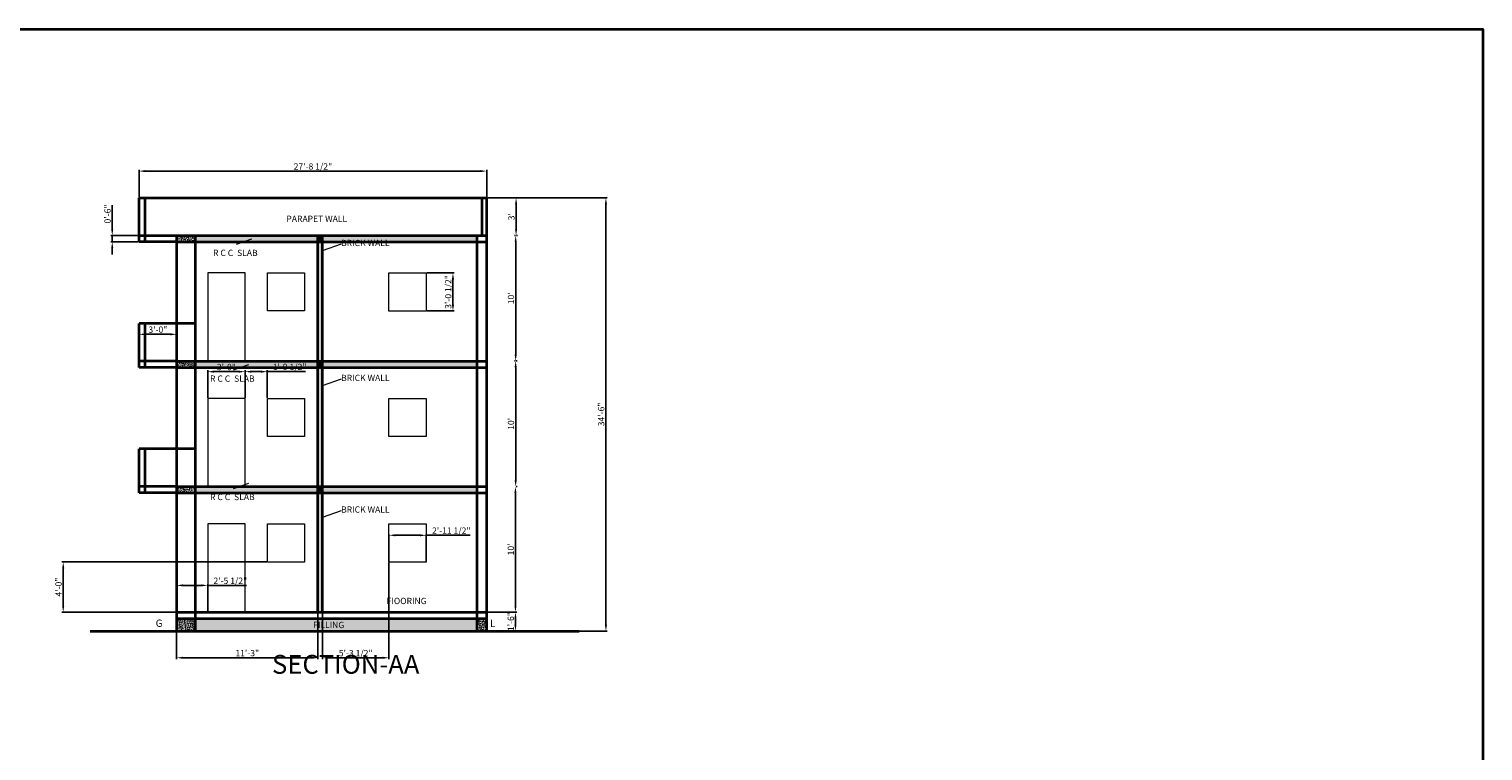
# Model space of a CAD drawing. Units: millimetres. Extents: x 50579 to 52843, y 62224 to 63803.
# Tile 5 of 5: x 51453 to 52843, y 63113 to 63803. Entities that reach past the tile are written whole.
import ezdxf

# ---------------------------------------------------------------- set-up
doc = ezdxf.new("R2010")
doc.units = ezdxf.units.MM
for name, color, linetype, lineweight in [('A-ANNO-DIMS', 2, 'Continuous', 18), ('A-ANNO-SYMB', 6, 'Continuous', 18), ('A-ANNO-TEXT', 6, 'Continuous', 18), ('A-ANNO-TITL', 4, 'Continuous', 25), ('A-ANNO-TTLB', 7, 'Continuous', 35), ('A-SECT', 7, 'Continuous', 35), ('A-SECT-OPEN', 7, 'Continuous', 18), ('A-SECT-PATT', 251, 'Continuous', 13)]:
    doc.layers.add(name, color=color, linetype=linetype, lineweight=lineweight)
doc.styles.get("Standard").update_dxf_attribs({"font": 'arial.ttf'})
doc.dimstyles.new('ISO-25', dxfattribs={"dimtxt": 6, "dimasz": 6, "dimexe": 1.25, "dimexo": 0.625, "dimtad": 1, "dimdec": 0, "dimlunit": 3, "dimtxsty": 'Standard', "dimcen": 2.5, "dimadec": 0, "dimazin": 0, "dimtfac": 1, "dimtdec": 0, "dimtmove": 0, "dimatfit": 3, "dimfxl": 1, "dimarcsym": 0})

# ---------------------------------------------------------------- blocks, each defined once
blk = doc.blocks.new('*D16')
at = {"layer": 'A-ANNO-DIMS', "color": 0, "lineweight": -2, "transparency": 16777216}
for p, q in [((51891, 63245.3), (51919.1, 63245.3)), ((51917.9, 63233.3), (51917.9, 63239.3)), ((51891, 63227.3), (51919.1, 63227.3))]:
    blk.add_line(p, q, dxfattribs=at)
at = {"layer": 'A-ANNO-DIMS', "color": 0, "transparency": 16777216}
for points in [[(51916.9, 63239.3), (51918.9, 63239.3), (51917.9, 63245.3)], [(51916.9, 63233.3), (51918.9, 63233.3), (51917.9, 63227.3)]]:
    blk.add_solid(points, dxfattribs=at)
at = {"layer": 'Defpoints', "color": 0, "transparency": 16777216}
for p in [(51890.4, 63245.3), (51917.9, 63245.3), (51890.4, 63227.3)]:
    blk.add_point(p, dxfattribs=at)
at = {"layer": 'A-ANNO-DIMS', "color": 0, "transparency": 16777216, "insert": (51914.2, 63236.3), "char_height": 6, "attachment_point": 5, "rotation": 90}
blk.add_mtext('1\'-6"', dxfattribs=at)
blk = doc.blocks.new('*D17')
at = {"layer": 'A-ANNO-DIMS', "color": 0, "lineweight": -2, "transparency": 16777216}
for p, q in [((51917.9, 63251.3), (51917.9, 63359.3)), ((51918.5, 63365.3), (51919.1, 63365.3)), ((51918.5, 63245.3), (51919.1, 63245.3))]:
    blk.add_line(p, q, dxfattribs=at)
at = {"layer": 'A-ANNO-DIMS', "color": 0, "transparency": 16777216}
for points in [[(51916.9, 63359.3), (51918.9, 63359.3), (51917.9, 63365.3)], [(51916.9, 63251.3), (51918.9, 63251.3), (51917.9, 63245.3)]]:
    blk.add_solid(points, dxfattribs=at)
at = {"layer": 'Defpoints', "color": 0, "transparency": 16777216}
for p in [(51917.9, 63365.3), (51917.9, 63365.3), (51917.9, 63245.3)]:
    blk.add_point(p, dxfattribs=at)
at = {"layer": 'A-ANNO-DIMS', "color": 0, "transparency": 16777216, "insert": (51914.2, 63305.3), "char_height": 6, "attachment_point": 5, "rotation": 90}
blk.add_mtext("10'", dxfattribs=at)
blk = doc.blocks.new('*D18')
at = {"layer": 'A-ANNO-DIMS', "color": 0, "lineweight": -2, "transparency": 16777216}
for p, q in [((51918.5, 63485.4), (51919.4, 63485.4)), ((51918.1, 63371.3), (51918.1, 63479.4)), ((51918.5, 63365.3), (51919.4, 63365.3))]:
    blk.add_line(p, q, dxfattribs=at)
at = {"layer": 'A-ANNO-DIMS', "color": 0, "transparency": 16777216}
for points in [[(51917.1, 63479.4), (51919.1, 63479.4), (51918.1, 63485.4)], [(51917.1, 63371.3), (51919.1, 63371.3), (51918.1, 63365.3)]]:
    blk.add_solid(points, dxfattribs=at)
at = {"layer": 'Defpoints', "color": 0, "transparency": 16777216}
for p in [(51917.9, 63485.4), (51918.1, 63485.4), (51917.9, 63365.3)]:
    blk.add_point(p, dxfattribs=at)
at = {"layer": 'A-ANNO-DIMS', "color": 0, "transparency": 16777216, "insert": (51914.4, 63425.3), "char_height": 6, "attachment_point": 5, "rotation": 90}
blk.add_mtext("10'", dxfattribs=at)
blk = doc.blocks.new('*D19')
at = {"layer": 'A-ANNO-DIMS', "color": 0, "lineweight": -2, "transparency": 16777216}
for p, q in [((51917.9, 63605.3), (51916.9, 63605.3)), ((51918.1, 63491.4), (51918.1, 63599.3)), ((51917.9, 63485.4), (51916.9, 63485.4))]:
    blk.add_line(p, q, dxfattribs=at)
at = {"layer": 'A-ANNO-DIMS', "color": 0, "transparency": 16777216}
for points in [[(51917.1, 63599.3), (51919.1, 63599.3), (51918.1, 63605.3)], [(51917.1, 63491.4), (51919.1, 63491.4), (51918.1, 63485.4)]]:
    blk.add_solid(points, dxfattribs=at)
at = {"layer": 'Defpoints', "color": 0, "transparency": 16777216}
for p in [(51918.1, 63605.3), (51918.5, 63605.3), (51918.5, 63485.4)]:
    blk.add_point(p, dxfattribs=at)
at = {"layer": 'A-ANNO-DIMS', "color": 0, "transparency": 16777216, "insert": (51914.4, 63545.3), "char_height": 6, "attachment_point": 5, "rotation": 90}
blk.add_mtext("10'", dxfattribs=at)
blk = doc.blocks.new('*D20')
at = {"layer": 'A-ANNO-DIMS', "color": 0, "lineweight": -2, "transparency": 16777216}
for p, q in [((51918.8, 63641.3), (51919.7, 63641.3)), ((51918.5, 63611.3), (51918.5, 63635.3)), ((51918.8, 63605.3), (51919.7, 63605.3))]:
    blk.add_line(p, q, dxfattribs=at)
at = {"layer": 'A-ANNO-DIMS', "color": 0, "transparency": 16777216}
for points in [[(51917.5, 63635.3), (51919.5, 63635.3), (51918.5, 63641.3)], [(51917.5, 63611.3), (51919.5, 63611.3), (51918.5, 63605.3)]]:
    blk.add_solid(points, dxfattribs=at)
at = {"layer": 'Defpoints', "color": 0, "transparency": 16777216}
for p in [(51918.1, 63641.3), (51918.5, 63641.3), (51918.1, 63605.3)]:
    blk.add_point(p, dxfattribs=at)
at = {"layer": 'A-ANNO-DIMS', "color": 0, "transparency": 16777216, "insert": (51914.8, 63623.3), "char_height": 6, "attachment_point": 5, "rotation": 90}
blk.add_mtext("3'", dxfattribs=at)
blk = doc.blocks.new('*D47')
at = {"layer": 'A-ANNO-DIMS', "color": 0, "lineweight": -2, "transparency": 16777216}
for p, q in [((51557.9, 63641.9), (51557.9, 63668.1)), ((51563.9, 63666.9), (51884.4, 63666.9)), ((51890.4, 63641.9), (51890.4, 63668.1))]:
    blk.add_line(p, q, dxfattribs=at)
at = {"layer": 'A-ANNO-DIMS', "color": 0, "transparency": 16777216}
for points in [[(51563.9, 63667.9), (51563.9, 63665.9), (51557.9, 63666.9)], [(51884.4, 63667.9), (51884.4, 63665.9), (51890.4, 63666.9)]]:
    blk.add_solid(points, dxfattribs=at)
at = {"layer": 'Defpoints', "color": 0, "transparency": 16777216}
for p in [(51890.4, 63666.9), (51557.9, 63641.3), (51890.4, 63641.3)]:
    blk.add_point(p, dxfattribs=at)
at = {"layer": 'A-ANNO-DIMS', "color": 0, "transparency": 16777216, "insert": (51724.2, 63670.6), "char_height": 6, "attachment_point": 5}
blk.add_mtext('27\'-8 1/2"', dxfattribs=at)
blk = doc.blocks.new('*D48')
at = {"layer": 'A-ANNO-DIMS', "color": 0, "lineweight": -2, "transparency": 16777216}
for p, q in [((51891, 63641.3), (52005.7, 63641.3)), ((52004.4, 63233.3), (52004.4, 63635.3)), ((51891, 63227.3), (52005.7, 63227.3))]:
    blk.add_line(p, q, dxfattribs=at)
at = {"layer": 'A-ANNO-DIMS', "color": 0, "transparency": 16777216}
for points in [[(52003.4, 63635.3), (52005.4, 63635.3), (52004.4, 63641.3)], [(52003.4, 63233.3), (52005.4, 63233.3), (52004.4, 63227.3)]]:
    blk.add_solid(points, dxfattribs=at)
at = {"layer": 'Defpoints', "color": 0, "transparency": 16777216}
for p in [(51890.4, 63641.3), (52004.4, 63641.3), (51890.4, 63227.3)]:
    blk.add_point(p, dxfattribs=at)
at = {"layer": 'A-ANNO-DIMS', "color": 0, "transparency": 16777216, "insert": (52000.7, 63434.3), "char_height": 6, "attachment_point": 5, "rotation": 90}
blk.add_mtext('34\'-6"', dxfattribs=at)
blk = doc.blocks.new('*D58')
at = {"layer": 'A-ANNO-DIMS', "color": 0, "lineweight": -2, "transparency": 16777216}
for p, q in [((51728.9, 63244.7), (51728.9, 63200.4)), ((51593.9, 63226.7), (51593.9, 63200.4)), ((51599.9, 63201.7), (51722.9, 63201.7))]:
    blk.add_line(p, q, dxfattribs=at)
at = {"layer": 'A-ANNO-DIMS', "color": 0, "transparency": 16777216}
for points in [[(51599.9, 63202.7), (51599.9, 63200.7), (51593.9, 63201.7)], [(51722.9, 63202.7), (51722.9, 63200.7), (51728.9, 63201.7)]]:
    blk.add_solid(points, dxfattribs=at)
at = {"layer": 'Defpoints', "color": 0, "transparency": 16777216}
for p in [(51728.9, 63245.3), (51593.9, 63227.3), (51728.9, 63201.7)]:
    blk.add_point(p, dxfattribs=at)
at = {"layer": 'A-ANNO-DIMS', "color": 0, "transparency": 16777216, "insert": (51661.4, 63205.4), "char_height": 6, "attachment_point": 5}
blk.add_mtext('11\'-3"', dxfattribs=at)
blk = doc.blocks.new('*D59')
at = {"layer": 'A-ANNO-DIMS', "color": 0, "lineweight": -2, "transparency": 16777216}
for p, q in [((51557.9, 63485.9), (51557.9, 63512.1)), ((51563.9, 63510.9), (51587.9, 63510.9)), ((51593.9, 63485.9), (51593.9, 63512.1))]:
    blk.add_line(p, q, dxfattribs=at)
at = {"layer": 'A-ANNO-DIMS', "color": 0, "transparency": 16777216}
for points in [[(51563.9, 63511.9), (51563.9, 63509.9), (51557.9, 63510.9)], [(51587.9, 63511.9), (51587.9, 63509.9), (51593.9, 63510.9)]]:
    blk.add_solid(points, dxfattribs=at)
at = {"layer": 'Defpoints', "color": 0, "transparency": 16777216}
for p in [(51593.9, 63510.9), (51557.9, 63485.3), (51593.9, 63485.3)]:
    blk.add_point(p, dxfattribs=at)
at = {"layer": 'A-ANNO-DIMS', "color": 0, "transparency": 16777216, "insert": (51575.9, 63514.6), "char_height": 6, "attachment_point": 5}
blk.add_mtext('3\'-0"', dxfattribs=at)
blk = doc.blocks.new('*D60')
at = {"layer": 'A-ANNO-DIMS', "color": 0, "lineweight": -2, "transparency": 16777216}
for p, q in [((51593.9, 63245.9), (51593.9, 63272.1)), ((51599.9, 63270.9), (51617.6, 63270.9)), ((51623.6, 63245.9), (51623.6, 63272.1)), ((51623.6, 63270.9), (51660.8, 63270.9))]:
    blk.add_line(p, q, dxfattribs=at)
at = {"layer": 'A-ANNO-DIMS', "color": 0, "transparency": 16777216}
for points in [[(51599.9, 63271.9), (51599.9, 63269.9), (51593.9, 63270.9)], [(51617.6, 63271.9), (51617.6, 63269.9), (51623.6, 63270.9)]]:
    blk.add_solid(points, dxfattribs=at)
at = {"layer": 'Defpoints', "color": 0, "transparency": 16777216}
for p in [(51623.6, 63270.9), (51593.9, 63245.3), (51623.6, 63245.3)]:
    blk.add_point(p, dxfattribs=at)
at = {"layer": 'A-ANNO-DIMS', "color": 0, "transparency": 16777216, "insert": (51645.2, 63274.6), "char_height": 6, "attachment_point": 5}
blk.add_mtext('2\'-5 1/2"', dxfattribs=at)
blk = doc.blocks.new('*D61')
at = {"layer": 'A-ANNO-DIMS', "color": 0, "lineweight": -2, "transparency": 16777216}
for p, q in [((51623.6, 63450.3), (51623.6, 63476.5)), ((51629.6, 63475.2), (51653.3, 63475.2)), ((51659.3, 63450.3), (51659.3, 63476.5))]:
    blk.add_line(p, q, dxfattribs=at)
at = {"layer": 'A-ANNO-DIMS', "color": 0, "transparency": 16777216}
for points in [[(51629.6, 63476.2), (51629.6, 63474.2), (51623.6, 63475.2)], [(51653.3, 63476.2), (51653.3, 63474.2), (51659.3, 63475.2)]]:
    blk.add_solid(points, dxfattribs=at)
at = {"layer": 'Defpoints', "color": 0, "transparency": 16777216}
for p in [(51659.3, 63475.2), (51623.6, 63449.6), (51659.3, 63449.6)]:
    blk.add_point(p, dxfattribs=at)
at = {"layer": 'A-ANNO-DIMS', "color": 0, "transparency": 16777216, "insert": (51641.4, 63478.9), "char_height": 6, "attachment_point": 5}
blk.add_mtext('3\'-0"', dxfattribs=at)
blk = doc.blocks.new('*D62')
at = {"layer": 'A-ANNO-DIMS', "color": 0, "lineweight": -2, "transparency": 16777216}
for p, q in [((51659.3, 63450.3), (51659.3, 63476.5)), ((51665.3, 63475.2), (51674.6, 63475.2)), ((51680.6, 63450.3), (51680.6, 63476.5)), ((51680.6, 63475.2), (51717.2, 63475.2))]:
    blk.add_line(p, q, dxfattribs=at)
at = {"layer": 'A-ANNO-DIMS', "color": 0, "transparency": 16777216}
for points in [[(51665.3, 63476.2), (51665.3, 63474.2), (51659.3, 63475.2)], [(51674.6, 63476.2), (51674.6, 63474.2), (51680.6, 63475.2)]]:
    blk.add_solid(points, dxfattribs=at)
at = {"layer": 'Defpoints', "color": 0, "transparency": 16777216}
for p in [(51680.6, 63475.2), (51659.3, 63449.6), (51680.6, 63449.6)]:
    blk.add_point(p, dxfattribs=at)
at = {"layer": 'A-ANNO-DIMS', "color": 0, "transparency": 16777216, "insert": (51701.9, 63479), "char_height": 6, "attachment_point": 5}
blk.add_mtext('1\'-9 1/2"', dxfattribs=at)
blk = doc.blocks.new('*D63')
at = {"layer": 'A-ANNO-DIMS', "color": 0, "lineweight": -2, "transparency": 16777216}
for p, q in [((51796.9, 63292.6), (51796.9, 63200.4)), ((51733.4, 63244.7), (51733.4, 63200.4)), ((51739.4, 63201.7), (51790.9, 63201.7))]:
    blk.add_line(p, q, dxfattribs=at)
at = {"layer": 'A-ANNO-DIMS', "color": 0, "transparency": 16777216}
for points in [[(51739.4, 63202.7), (51739.4, 63200.7), (51733.4, 63201.7)], [(51790.9, 63202.7), (51790.9, 63200.7), (51796.9, 63201.7)]]:
    blk.add_solid(points, dxfattribs=at)
at = {"layer": 'Defpoints', "color": 0, "transparency": 16777216}
for p in [(51796.9, 63293.2), (51733.4, 63245.3), (51796.9, 63201.7)]:
    blk.add_point(p, dxfattribs=at)
at = {"layer": 'A-ANNO-DIMS', "color": 0, "transparency": 16777216, "insert": (51765.1, 63205.4), "char_height": 6, "attachment_point": 5}
blk.add_mtext('5\'-3 1/2"', dxfattribs=at)
blk = doc.blocks.new('*D64')
at = {"layer": 'A-ANNO-DIMS', "color": 0, "lineweight": -2, "transparency": 16777216}
for p, q in [((51796.9, 63293.8), (51796.9, 63320)), ((51802.9, 63318.8), (51826.5, 63318.8)), ((51832.5, 63293.8), (51832.5, 63320)), ((51832.5, 63318.8), (51874.5, 63318.8))]:
    blk.add_line(p, q, dxfattribs=at)
at = {"layer": 'A-ANNO-DIMS', "color": 0, "transparency": 16777216}
for points in [[(51802.9, 63319.8), (51802.9, 63317.8), (51796.9, 63318.8)], [(51826.5, 63319.8), (51826.5, 63317.8), (51832.5, 63318.8)]]:
    blk.add_solid(points, dxfattribs=at)
at = {"layer": 'Defpoints', "color": 0, "transparency": 16777216}
for p in [(51832.5, 63318.8), (51796.9, 63293.2), (51832.5, 63293.2)]:
    blk.add_point(p, dxfattribs=at)
at = {"layer": 'A-ANNO-DIMS', "color": 0, "transparency": 16777216, "insert": (51856.5, 63322.5), "char_height": 6, "attachment_point": 5}
blk.add_mtext('2\'-11 1/2"', dxfattribs=at)
blk = doc.blocks.new('*D65')
at = {"layer": 'A-ANNO-DIMS', "color": 0, "lineweight": -2, "transparency": 16777216}
for p, q in [((51833.1, 63569.6), (51859.4, 63569.6)), ((51858.1, 63563.6), (51858.1, 63539.2)), ((51833.1, 63533.2), (51859.4, 63533.2))]:
    blk.add_line(p, q, dxfattribs=at)
at = {"layer": 'A-ANNO-DIMS', "color": 0, "transparency": 16777216}
for points in [[(51857.1, 63563.6), (51859.1, 63563.6), (51858.1, 63569.6)], [(51857.1, 63539.2), (51859.1, 63539.2), (51858.1, 63533.2)]]:
    blk.add_solid(points, dxfattribs=at)
at = {"layer": 'Defpoints', "color": 0, "transparency": 16777216}
for p in [(51832.5, 63569.6), (51832.5, 63533.2), (51858.1, 63533.2)]:
    blk.add_point(p, dxfattribs=at)
at = {"layer": 'A-ANNO-DIMS', "color": 0, "transparency": 16777216, "insert": (51854.4, 63551.4), "char_height": 6, "attachment_point": 5, "rotation": 90}
blk.add_mtext('3\'-0 1/2"', dxfattribs=at)
blk = doc.blocks.new('*D66')
at = {"layer": 'A-ANNO-DIMS', "color": 0, "lineweight": -2, "transparency": 16777216}
for p, q in [((51680, 63293.3), (51484.2, 63293.3)), ((51485.4, 63287.3), (51485.4, 63251.3)), ((51658.7, 63245.3), (51484.2, 63245.3))]:
    blk.add_line(p, q, dxfattribs=at)
at = {"layer": 'A-ANNO-DIMS', "color": 0, "transparency": 16777216}
for points in [[(51484.4, 63287.3), (51486.4, 63287.3), (51485.4, 63293.3)], [(51484.4, 63251.3), (51486.4, 63251.3), (51485.4, 63245.3)]]:
    blk.add_solid(points, dxfattribs=at)
at = {"layer": 'Defpoints', "color": 0, "transparency": 16777216}
for p in [(51680.6, 63293.3), (51485.4, 63245.3), (51659.3, 63245.3)]:
    blk.add_point(p, dxfattribs=at)
at = {"layer": 'A-ANNO-DIMS', "color": 0, "transparency": 16777216, "insert": (51481.7, 63269.3), "char_height": 6, "attachment_point": 5, "rotation": 90}
blk.add_mtext('4\'-0"', dxfattribs=at)
blk = doc.blocks.new('*D67')
at = {"layer": 'A-ANNO-DIMS', "color": 0, "lineweight": -2, "transparency": 16777216}
for p, q in [((51532.3, 63611.3), (51532.3, 63634.5)), ((51557.3, 63605.3), (51531.1, 63605.3)), ((51557.3, 63599.3), (51531.1, 63599.3)), ((51532.3, 63599.3), (51532.3, 63605.3)), ((51532.3, 63593.3), (51532.3, 63587.3))]:
    blk.add_line(p, q, dxfattribs=at)
at = {"layer": 'A-ANNO-DIMS', "color": 0, "transparency": 16777216}
for points in [[(51531.3, 63611.3), (51533.3, 63611.3), (51532.3, 63605.3)], [(51531.3, 63593.3), (51533.3, 63593.3), (51532.3, 63599.3)]]:
    blk.add_solid(points, dxfattribs=at)
at = {"layer": 'Defpoints', "color": 0, "transparency": 16777216}
for p in [(51532.3, 63605.3), (51557.9, 63605.3), (51557.9, 63599.3)]:
    blk.add_point(p, dxfattribs=at)
at = {"layer": 'A-ANNO-DIMS', "color": 0, "transparency": 16777216, "insert": (51528.6, 63625.9), "char_height": 6, "attachment_point": 5, "rotation": 90}
blk.add_mtext('0\'-6"', dxfattribs=at)

msp = doc.modelspace()

# ---------------------------------------------------------------- hatches: boundary and pattern name
at = {"layer": 'A-SECT-PATT'}
h = msp.add_hatch(dxfattribs=at)
h.set_pattern_fill('AR-CONC', color=256, scale=0.01)
h.paths.add_polyline_path([(51611.8, 63605.28), (51593.92, 63605.28), (51593.92, 63599.28), (51611.8, 63599.28)])
h = msp.add_hatch(dxfattribs=at)
h.set_pattern_fill('AR-CONC', color=256, scale=0.01)
h.paths.add_polyline_path([(51728.92, 63605.28), (51611.8, 63605.28), (51611.8, 63599.28), (51728.92, 63599.28)])
h = msp.add_hatch(dxfattribs=at)
h.set_pattern_fill('BRICK', color=256, scale=0.01)
h.paths.add_polyline_path([(51733.42, 63605.28), (51728.92, 63605.28), (51728.92, 63599.28), (51733.42, 63599.28)])
h = msp.add_hatch(dxfattribs=at)
h.set_pattern_fill('BRICK', color=256, scale=0.01)
h.paths.add_polyline_path([(51733.42, 63599.28), (51728.92, 63599.28), (51728.92, 63485.28), (51733.42, 63485.28)])
h = msp.add_hatch(dxfattribs=at)
h.set_pattern_fill('AR-CONC', color=256, scale=0.01)
h.paths.add_polyline_path([(51881.42, 63605.28), (51733.42, 63605.28), (51733.42, 63599.28), (51881.42, 63599.28)])
h = msp.add_hatch(dxfattribs=at)
h.set_pattern_fill('AR-CONC', color=256, scale=0.01)
h.paths.add_polyline_path([(51611.8, 63485.28), (51593.92, 63485.28), (51593.92, 63479.28), (51611.8, 63479.28)])
h = msp.add_hatch(dxfattribs=at)
h.set_pattern_fill('AR-CONC', color=256, scale=0.01)
h.paths.add_polyline_path([(51728.92, 63485.28), (51611.8, 63485.28), (51611.8, 63479.28), (51728.92, 63479.28)])
h = msp.add_hatch(dxfattribs=at)
h.set_pattern_fill('BRICK', color=256, scale=0.01)
h.paths.add_polyline_path([(51733.42, 63485.28), (51728.92, 63485.28), (51728.92, 63479.28), (51733.42, 63479.28)])
h = msp.add_hatch(dxfattribs=at)
h.set_pattern_fill('AR-CONC', color=256, scale=0.01)
h.paths.add_polyline_path([(51881.42, 63485.28), (51733.42, 63485.28), (51733.42, 63479.28), (51881.42, 63479.28)])
h = msp.add_hatch(dxfattribs=at)
h.set_pattern_fill('BRICK', color=256, scale=0.01)
h.paths.add_polyline_path([(51733.42, 63479.28), (51728.92, 63479.28), (51728.92, 63365.28), (51733.42, 63365.28)])
h = msp.add_hatch(dxfattribs=at)
h.set_pattern_fill('AR-CONC', color=256, scale=0.01)
h.paths.add_polyline_path([(51611.8, 63365.28), (51593.92, 63365.28), (51593.92, 63359.28), (51611.8, 63359.28)])
h = msp.add_hatch(dxfattribs=at)
h.set_pattern_fill('AR-CONC', color=256, scale=0.01)
h.paths.add_polyline_path([(51728.92, 63365.28), (51611.8, 63365.28), (51611.8, 63359.28), (51728.92, 63359.28)])
h = msp.add_hatch(dxfattribs=at)
h.set_pattern_fill('BRICK', color=256, scale=0.01)
h.paths.add_polyline_path([(51733.42, 63365.28), (51728.92, 63365.28), (51728.92, 63359.28), (51733.42, 63359.28)])
h = msp.add_hatch(dxfattribs=at)
h.set_pattern_fill('BRICK', color=256, scale=0.01)
h.paths.add_polyline_path([(51733.42, 63359.28), (51728.92, 63359.28), (51728.92, 63245.28), (51733.42, 63245.28)])
h = msp.add_hatch(dxfattribs=at)
h.set_pattern_fill('AR-CONC', color=256, scale=0.01)
h.paths.add_polyline_path([(51881.42, 63365.28), (51733.42, 63365.28), (51733.42, 63359.28), (51881.42, 63359.28)])
h = msp.add_hatch(dxfattribs=at)
h.set_pattern_fill('AR-CONC', color=256, scale=0.01)
h.paths.add_polyline_path([(51611.8, 63239.28), (51593.92, 63239.28), (51593.92, 63227.28), (51611.8, 63227.28)])
h = msp.add_hatch(dxfattribs=at)
h.set_pattern_fill('AR-CONC', color=256, scale=0.01)
h.paths.add_polyline_path([(51881.42, 63239.28), (51611.8, 63239.28), (51611.8, 63227.28), (51881.42, 63227.28)])
h = msp.add_hatch(dxfattribs=at)
h.set_pattern_fill('AR-CONC', color=256, scale=0.01)
h.paths.add_polyline_path([(51890.42, 63239.28), (51881.42, 63239.28), (51881.42, 63227.28), (51890.42, 63227.28)])

# ---------------------------------------------------------------- linework, layer by layer
at = {"layer": 'A-ANNO-TEXT'}
for p, q in [((51665.37, 63601.77), (51650.75, 63596.65)), ((51733.42, 63590.88), (51751.68, 63597.27)), ((51662.51, 63481.59), (51647.89, 63476.47)), ((51733.42, 63461.89), (51751.68, 63468.29)), ((51662.51, 63368.43), (51647.89, 63363.31)), ((51733.42, 63336.09), (51751.68, 63342.48))]:
    msp.add_line(p, q, dxfattribs=at)
at = {"layer": 'A-ANNO-TTLB'}
msp.add_lwpolyline([(50579.46, 63802.65), (52843.1, 63802.65), (52843.1, 62224.04), (50579.46, 62224.04)], close=True, dxfattribs=at)
at = {"layer": 'A-SECT'}
for p, q in [((51557.92, 63599.28), (51557.92, 63641.28)), ((51557.92, 63641.28), (51890.42, 63641.28)), ((51563.92, 63599.28), (51563.92, 63641.28)), ((51885.92, 63605.28), (51885.92, 63641.28)), ((51890.42, 63227.28), (51890.42, 63641.28)), ((51557.92, 63605.28), (51890.42, 63605.28)), ((51593.92, 63599.28), (51557.92, 63599.28)), ((51593.92, 63227.28), (51593.92, 63605.28)), ((51593.92, 63599.28), (51890.42, 63599.28)), ((51611.8, 63227.28), (51611.8, 63605.28)), ((51728.92, 63245.28), (51728.92, 63605.28)), ((51733.42, 63245.28), (51733.42, 63605.28)), ((51881.42, 63227.28), (51881.42, 63605.28)), ((51557.92, 63479.28), (51557.92, 63521.28)), ((51611.8, 63521.28), (51557.92, 63521.28)), ((51563.92, 63479.28), (51563.92, 63521.28)), ((51593.92, 63485.28), (51557.92, 63485.28)), ((51593.92, 63485.28), (51890.42, 63485.28)), ((51593.92, 63479.28), (51557.92, 63479.28)), ((51593.92, 63479.28), (51890.42, 63479.28)), ((51557.92, 63359.28), (51557.92, 63401.28)), ((51611.8, 63401.28), (51557.92, 63401.28)), ((51563.92, 63359.28), (51563.92, 63401.28)), ((51593.92, 63365.28), (51557.92, 63365.28)), ((51593.92, 63359.28), (51557.92, 63359.28)), ((51593.92, 63365.28), (51890.42, 63365.28)), ((51593.92, 63359.28), (51890.42, 63359.28)), ((51593.92, 63245.28), (51890.42, 63245.28)), ((51593.92, 63239.28), (51890.42, 63239.28)), ((51511.03, 63227.28), (51978.82, 63227.28))]:
    msp.add_line(p, q, dxfattribs=at)
at = {"layer": 'A-SECT-OPEN'}
for points in [[(51623.56, 63485.28), (51659.31, 63485.28), (51659.31, 63569.63), (51623.56, 63569.63)], [(51680.63, 63569.63), (51716.01, 63569.63), (51716.01, 63533.26), (51680.63, 63533.26)], [(51796.88, 63569.63), (51832.52, 63569.63), (51832.52, 63533.18), (51796.88, 63533.18)], [(51623.56, 63365.28), (51659.31, 63365.28), (51659.31, 63449.63), (51623.56, 63449.63)], [(51680.63, 63449.63), (51716.01, 63449.63), (51716.01, 63413.26), (51680.63, 63413.26)], [(51796.88, 63449.63), (51832.52, 63449.63), (51832.52, 63413.18), (51796.88, 63413.18)], [(51623.56, 63245.28), (51659.31, 63245.28), (51659.31, 63329.63), (51623.56, 63329.63)], [(51680.63, 63329.63), (51716.01, 63329.63), (51716.01, 63293.26), (51680.63, 63293.26)], [(51796.88, 63329.63), (51832.52, 63329.63), (51832.52, 63293.18), (51796.88, 63293.18)]]:
    msp.add_lwpolyline(points, close=True, dxfattribs=at)

# ---------------------------------------------------------------- texts
at = {"layer": 'A-ANNO-SYMB', "char_height": 7, "attachment_point": 1}
for s, insert in [('  G', (51569.56, 63238.26)), ('  L', (51889.22, 63238.04))]:
    msp.add_mtext_dynamic_manual_height_columns(s, width=13.8936, gutter_width=12.5, heights=[0], dxfattribs=dict(at, insert=insert))
at = {"layer": 'A-ANNO-TEXT', "char_height": 6, "attachment_point": 1}
for s, insert in [('    PARAPET WALL', (51691.47, 63624.29)), ('   BRICK WALL', (51745.63, 63601.21)), ('    R C C  SLAB', (51621.36, 63591.73)), ('    R C C  SLAB', (51618.5, 63471.55)), ('   BRICK WALL', (51745.63, 63472.23)), ('    R C C  SLAB', (51618.5, 63358.39)), ('   BRICK WALL', (51745.63, 63346.42)), ('    FIOORING', (51787.36, 63259.02)), ('    FILLING', (51717.07, 63236.08))]:
    msp.add_mtext_dynamic_manual_height_columns(s, width=88.9546, gutter_width=12.5, heights=[0], dxfattribs=dict(at, insert=insert))
at = {"layer": 'A-ANNO-TITL', "insert": (51674.06, 63204.47), "char_height": 18, "attachment_point": 1}
msp.add_mtext_dynamic_manual_height_columns('  SECTION-AA', width=341.9217, gutter_width=12.5, heights=[0], dxfattribs=at)

# ---------------------------------------------------------------- dimensions: what is measured, and where the dimension line sits
at = {"layer": 'A-ANNO-DIMS'}
for base, p1, p2, picture, middle in [((51890.42, 63666.88), (51557.92, 63641.28), (51890.42, 63641.28), '*D47', (51724.17, 63670.61)), ((51593.92, 63510.88), (51557.92, 63485.28), (51593.92, 63485.28), '*D59', (51575.92, 63514.57)), ((51659.3082, 63475.225), (51623.5577, 63449.625), (51659.3082, 63449.625), '*D61', (51641.433, 63478.9155)), ((51680.63, 63475.23), (51659.31, 63449.63), (51680.63, 63449.63), '*D62', (51701.93, 63478.95)), ((51832.52, 63318.78), (51796.88, 63293.18), (51832.52, 63293.18), '*D64', (51856.5, 63322.51)), ((51796.88, 63201.68), (51733.42, 63245.28), (51796.88, 63293.18), '*D63', (51765.15, 63205.41)), ((51623.56, 63270.88), (51593.92, 63245.28), (51623.56, 63245.28), '*D60', (51645.2, 63274.61)), ((51728.92, 63201.68), (51593.92, 63227.28), (51728.92, 63245.28), '*D58', (51661.42, 63205.37))]:
    dim = msp.add_linear_dim(base=base, p1=p1, p2=p2, dimstyle='ISO-25', override={"dimdec": 1, "dimlfac": 1, "dimrnd": 0, "dimzin": 1, "dimdsep": 46, "dimlunit": 4, "dimfrac": 2}, dxfattribs=at)
    dim.commit()
    dim.dimension.update_dxf_attribs({"geometry": picture, "text_midpoint": middle})
for base, p1, p2, angle, override, picture, middle in [((52004.42, 63641.28), (51890.42, 63227.28), (51890.42, 63641.28), 90, {"dimdec": 1, "dimlfac": 1, "dimrnd": 0, "dimzin": 1, "dimdsep": 46, "dimlunit": 4, "dimfrac": 2}, '*D48', (52000.73, 63434.28)), ((51918.5, 63641.28), (51918.13, 63605.28), (51918.13, 63641.28), 90, {"dimclrd": 0, "dimclre": 0, "dimclrt": 0}, '*D20', (51914.81, 63623.28)), ((51532.32, 63605.28), (51557.92, 63599.28), (51557.92, 63605.28), 90, {"dimdec": 1, "dimlfac": 1, "dimrnd": 0, "dimzin": 1, "dimdsep": 46, "dimlunit": 4, "dimfrac": 2}, '*D67', (51528.63, 63625.88)), ((51918.13, 63605.28), (51918.5, 63485.36), (51918.5, 63605.28), 90, {"dimclrd": 0, "dimclre": 0, "dimclrt": 0}, '*D19', (51914.44, 63545.32)), ((51858.1232, 63533.184), (51832.5232, 63569.625), (51832.5232, 63533.184), 270, {"dimdec": 1, "dimlfac": 1, "dimrnd": 0, "dimzin": 1, "dimdsep": 46, "dimlunit": 4, "dimfrac": 2}, '*D65', (51854.3938, 63551.4045)), ((51918.13, 63485.36), (51917.87, 63365.28), (51917.87, 63485.36), 90, {"dimclrd": 0, "dimclre": 0, "dimclrt": 0}, '*D18', (51914.44, 63425.32)), ((51917.87, 63365.28), (51917.87, 63245.28), (51917.87, 63365.28), 90, {"dimclrd": 0, "dimclre": 0, "dimclrt": 0}, '*D17', (51914.19, 63305.28)), ((51485.43, 63245.28), (51680.63, 63293.26), (51659.31, 63245.28), 90, {"dimdec": 1, "dimlfac": 1, "dimrnd": 0, "dimzin": 1, "dimdsep": 46, "dimlunit": 4, "dimfrac": 2}, '*D66', (51481.74, 63269.27)), ((51917.87, 63245.28), (51890.42, 63227.28), (51890.42, 63245.28), 90, {"dimclrd": 0, "dimclre": 0, "dimclrt": 0}, '*D16', (51914.19, 63236.28))]:
    dim = msp.add_linear_dim(base=base, p1=p1, p2=p2, angle=angle, dimstyle='ISO-25', override=override, dxfattribs=at)
    dim.commit()
    dim.dimension.update_dxf_attribs({"geometry": picture, "text_midpoint": middle})

doc.saveas('drawing.dxf')
